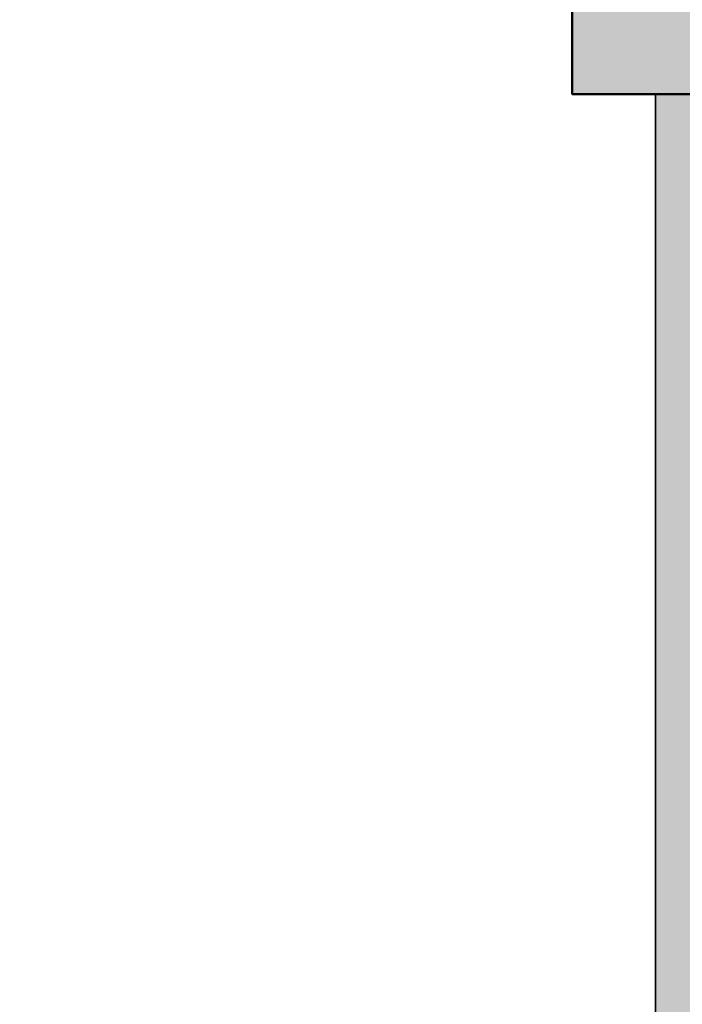
# Model space of a CAD drawing. Units: inches. Extents: x 1998 to 2588, y 1139 to 1977.
# Tile 57 of 134: x 2288 to 2344, y 1663 to 1746. Entities that reach past the tile are written whole.
import ezdxf

# ---------------------------------------------------------------- set-up
doc = ezdxf.new("R2010")
doc.units = ezdxf.units.IN
for name, color, linetype, lineweight in [('A-COLS-PATT', 250, 'Continuous', 13), ('A-WALL-PATT', 252, 'Continuous', 13), ('COLUMN', 10, 'Continuous', 50), ('WALL', 200, 'Continuous', 35)]:
    doc.layers.add(name, color=color, linetype=linetype, lineweight=lineweight)

msp = doc.modelspace()

# ---------------------------------------------------------------- hatches: boundary and pattern name
at = {"layer": 'A-COLS-PATT'}
h = msp.add_hatch(color=256, dxfattribs=at)
h.dxf.hatch_style = 1
h.paths.add_polyline_path([(2099.4125, 1888.7324), (2087.9729, 1888.7324), (2087.9729, 1868.3278), (2099.4125, 1868.3278)])
h.paths.add_polyline_path([(2234.4125, 1888.7324), (2222.9729, 1888.7324), (2222.9729, 1868.3278), (2234.4125, 1868.3278)])
h.paths.add_polyline_path([(2341.4729, 1886.637), (2330.0332, 1886.637), (2330.0332, 1866.2324), (2341.4729, 1866.2324)])
h.paths.add_polyline_path([(2507.8006, 1882.7324), (2487.396, 1882.7324), (2487.396, 1871.2927), (2507.8006, 1871.2927)])
h.paths.add_polyline_path([(2510.9729, 1766.672), (2490.5682, 1766.672), (2490.5682, 1755.2324), (2510.9729, 1755.2324)])
h.paths.add_polyline_path([(2345.9729, 1759.7324), (2334.5332, 1759.7324), (2334.5332, 1739.3278), (2345.9729, 1739.3278)])
h.paths.add_polyline_path([(2234.4125, 1774.3318), (2222.9729, 1774.3318), (2222.9729, 1753.9272), (2234.4125, 1753.9272)])
h.paths.add_polyline_path([(2099.4125, 1775.637), (2087.9729, 1775.637), (2087.9729, 1755.2324), (2099.4125, 1755.2324)])
h.paths.add_polyline_path([(2098.0956, 1593.7241), (2077.691, 1593.7241), (2077.691, 1582.2845), (2098.0956, 1582.2845)])
h.paths.add_polyline_path([(2227.4729, 1604.637), (2216.0332, 1604.637), (2216.0332, 1584.2324), (2227.4729, 1584.2324)])
h.paths.add_polyline_path([(2345.9729, 1647.5211), (2334.5332, 1647.5211), (2334.5332, 1627.1165), (2345.9729, 1627.1165)])
h.paths.add_polyline_path([(2522.3775, 1641.2324), (2501.9729, 1641.2324), (2501.9729, 1629.7927), (2522.3775, 1629.7927)])
h.paths.add_polyline_path([(2522.3775, 1480.7324), (2501.9729, 1480.7324), (2501.9729, 1469.2927), (2522.3775, 1469.2927)])
h.paths.add_polyline_path([(2345.9729, 1488.5616), (2334.5332, 1488.5616), (2334.5332, 1468.1569), (2345.9729, 1468.1569)])
h.paths.add_polyline_path([(2234.4125, 1486.137), (2227.4729, 1486.137), (2227.4729, 1465.7324), (2234.4125, 1465.7324)])
h.paths.add_polyline_path([(2227.4729, 1486.137), (2222.9729, 1486.137), (2222.9729, 1465.7324), (2227.4729, 1465.7324)])
h.paths.add_polyline_path([(2108.3775, 1470.2324), (2087.9729, 1470.2324), (2087.9729, 1458.7927), (2108.3775, 1458.7927)])
h.paths.add_polyline_path([(2096.9729, 1365.5012), (2087.9729, 1365.5012), (2087.9729, 1345.0966), (2096.9729, 1345.0966)])
h.paths.add_polyline_path([(2087.9729, 1365.5012), (2085.5332, 1365.5012), (2085.5332, 1345.0966), (2087.9729, 1345.0966)])
h.paths.add_polyline_path([(2234.4125, 1285.137), (2222.9729, 1285.137), (2222.9729, 1264.7324), (2234.4125, 1264.7324)])
h.paths.add_polyline_path([(2345.9729, 1285.137), (2334.5332, 1285.137), (2334.5332, 1264.7324), (2345.9729, 1264.7324)])
h.paths.add_polyline_path([(2503.1458, 1240.172), (2482.7412, 1240.172), (2482.7412, 1228.7324), (2503.1458, 1228.7324)])
h.paths.add_polyline_path([(2510.9729, 1369.172), (2490.5682, 1369.172), (2490.5682, 1357.7324), (2510.9729, 1357.7324)])
at = {"layer": 'A-WALL-PATT'}
h = msp.add_hatch(color=256, dxfattribs=at)
h.dxf.hatch_style = 1
h.paths.add_polyline_path([(2527.4729, 1362.2324), (2510.9729, 1362.2324), (2510.9729, 1357.7324), (2518.4729, 1357.7324), (2518.4729, 1237.7324), (2503.1458, 1237.7324), (2503.1458, 1228.7324), (2527.4729, 1228.7324)])
h.paths.add_polyline_path([(2490.5682, 1362.2324), (2398.4729, 1362.2324), (2398.4729, 1357.7324), (2490.5682, 1357.7324)])
h.paths.add_polyline_path([(2224.9729, 1264.7324), (2222.9729, 1264.7324), (2222.9729, 1232.4125), (2341.4729, 1232.4125), (2341.4729, 1234.4125), (2224.9729, 1234.4125)])
h.paths.add_polyline_path([(2334.5332, 1273.7324), (2264.7638, 1273.7324), (2264.7638, 1269.5611, -0.043659), (2264.3413, 1264.7324), (2334.5332, 1264.7324)])
h.paths.add_polyline_path([(2236.9551, 1273.7324), (2234.4125, 1273.7324), (2234.4125, 1264.7324), (2236.9551, 1264.7324), (2236.9551, 1269.5611)])
h.paths.add_polyline_path([(2222.9729, 1293.2324), (2096.9729, 1293.2324), (2096.9729, 1345.0966), (2087.9729, 1345.0966), (2087.9729, 1284.2324), (2222.9729, 1284.2324), (2222.9729, 1285.137)])
h.paths.add_polyline_path([(2096.9729, 1458.7927), (2087.9729, 1458.7927), (2087.9729, 1417.7324), (2087.9729, 1413.2324), (2096.9729, 1413.2324), (2096.9729, 1417.7324)])
h.paths.add_polyline_path([(2096.9729, 1413.2324), (2087.9729, 1413.2324), (2087.9729, 1365.5012), (2096.9729, 1365.5012), (2096.9729, 1369.3358)])
h.paths.add_polyline_path([(2186.2943, 1417.7324), (2138.6074, 1417.7324), (2096.9729, 1417.7324), (2096.9729, 1413.2324), (2138.6074, 1413.2324), (2186.2943, 1413.2324)])
h.paths.add_polyline_path([(2181.4729, 1465.7324), (2176.9729, 1465.7324), (2176.9729, 1451.6434), (2181.4729, 1451.6434)])
h.paths.add_polyline_path([(2181.4729, 1422.1664), (2176.9729, 1422.1664), (2176.9729, 1417.7324), (2181.4729, 1417.7324)])
h.paths.add_polyline_path([(2063.9729, 1465.7324), (2087.9729, 1465.7324), (2087.9729, 1470.2324), (2059.4729, 1470.2324), (2059.4729, 1413.2324), (2087.9729, 1413.2324), (2087.9729, 1417.7324), (2063.9729, 1417.7324)])
h.paths.add_polyline_path([(2181.4729, 1755.2324), (2176.9729, 1755.2324), (2176.9729, 1748.6798), (2177.0513, 1748.6798), (2181.4729, 1748.6798)])
h.paths.add_polyline_path([(2227.4729, 1707.2324), (2220.4647, 1707.2324), (2220.4647, 1702.7324), (2222.9729, 1702.7324), (2222.9729, 1604.637), (2227.4729, 1604.637)])
h.paths.add_polyline_path([(2114.9729, 1702.7324), (2105.9729, 1702.7324), (2105.9729, 1628.4781, -0.0318759), (2110.1012, 1628.7416), (2114.9729, 1628.7416)])
h.paths.add_polyline_path([(2345.9729, 1739.3278), (2341.4729, 1739.3278), (2341.4729, 1647.5211), (2345.9729, 1647.5211)])
h.paths.add_polyline_path([(2350.6273, 1641.2324), (2345.9729, 1641.2324), (2345.9729, 1636.7324), (2350.6273, 1636.7324), (2350.6273, 1639.8729)])
h.paths.add_polyline_path([(2501.9729, 1641.2324), (2407.9729, 1641.2324), (2392.5005, 1641.2324), (2392.5005, 1639.8729), (2392.5005, 1636.7324), (2501.9729, 1636.7324)])
h.paths.add_polyline_path([(2510.9729, 1755.2324), (2501.9729, 1755.2324), (2501.9729, 1641.2324), (2510.9729, 1641.2324)])
h.paths.add_polyline_path([(2549.1786, 1641.2324), (2522.3775, 1641.2324), (2522.3775, 1636.7324), (2540.1786, 1636.7324), (2540.1786, 1480.7324), (2522.3775, 1480.7324), (2522.3775, 1476.2324), (2549.1786, 1476.2324)])
h.paths.add_polyline_path([(2498.1786, 1594.7324), (2407.9729, 1594.7324), (2407.9729, 1585.7324), (2416.9729, 1585.7324), (2489.1786, 1585.7324), (2489.1786, 1531.7324), (2416.9729, 1531.7324), (2407.9729, 1531.7324), (2407.9729, 1522.7324), (2498.1786, 1522.7324)])
h.paths.add_polyline_path([(2351.6437, 1480.7324), (2345.9729, 1480.7324), (2345.9729, 1476.2324), (2351.6437, 1476.2324), (2351.6437, 1477.5919)])
h.paths.add_polyline_path([(2501.9729, 1480.7324), (2498.1786, 1480.7324), (2407.9729, 1480.7324), (2393.5168, 1480.7324), (2393.5168, 1477.5919), (2393.5168, 1476.2324), (2501.9729, 1476.2324)])

# ---------------------------------------------------------------- linework, layer by layer
at = {"layer": 'COLUMN'}
msp.add_lwpolyline([(2334.5332, 1759.7324), (2345.9729, 1759.7324), (2345.9729, 1739.3278), (2334.5332, 1739.3278)], close=True, dxfattribs=at)
at = {"layer": 'WALL'}
msp.add_line((2341.4729, 1739.3278), (2341.4729, 1647.5211), dxfattribs=at)

doc.saveas('drawing.dxf')
